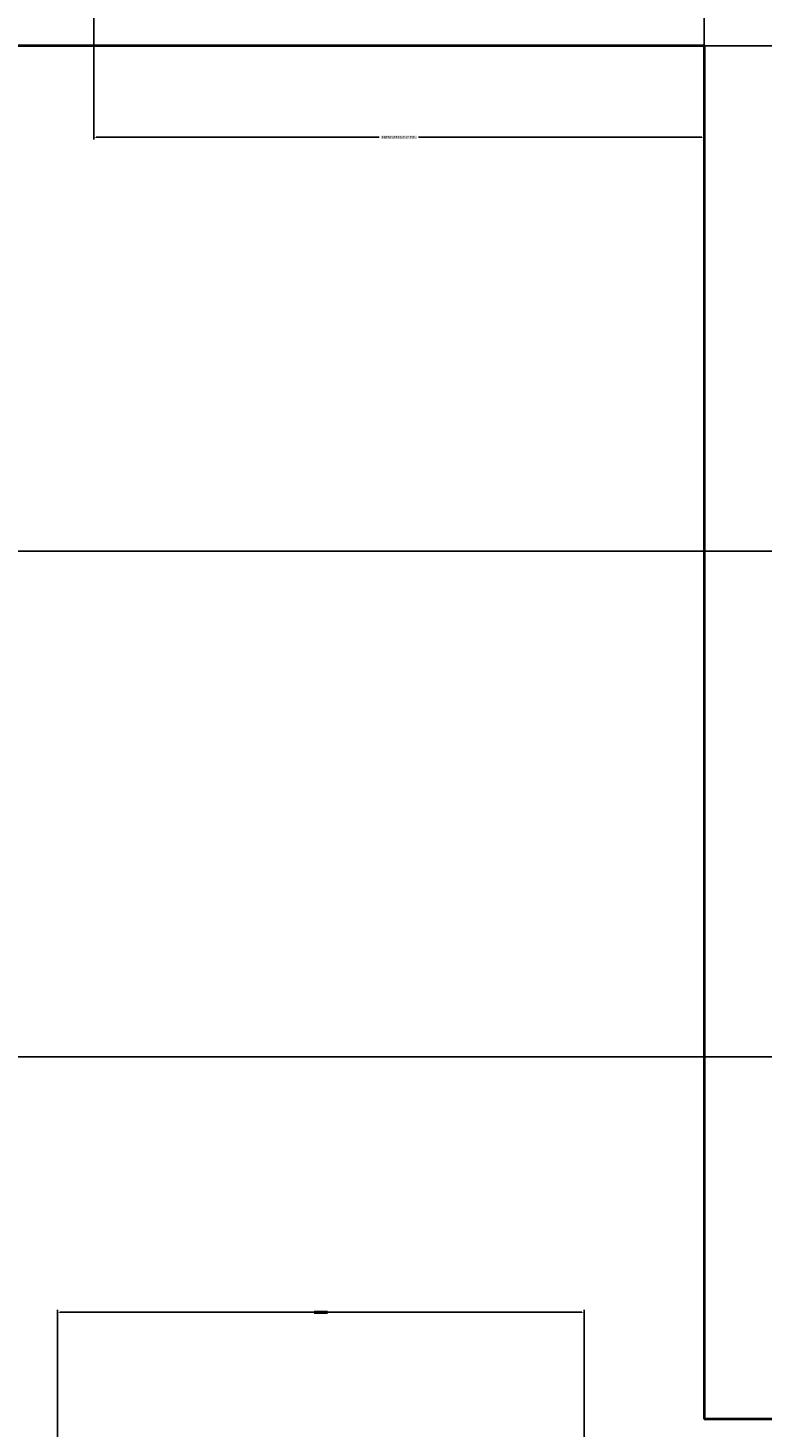
# Model space of a CAD drawing. Units: inches. Extents: x -301 to 715, y -607 to 364.
# Tile 117 of 141: x -43 to 14, y 192 to 303. Entities that reach past the tile are written whole.
import ezdxf

# ---------------------------------------------------------------- set-up
doc = ezdxf.new("R2010")
doc.units = ezdxf.units.IN
doc.header["$MEASUREMENT"] = 0
for name, color, linetype, lineweight in [('A-ANNO-DIMS', 2, 'Continuous', 18), ('A-FLOR-STRS', 2, 'Continuous', 25), ('A-WALL', 3, 'Continuous', 40)]:
    doc.layers.add(name, color=color, linetype=linetype, lineweight=lineweight)
doc.styles.get("Standard").update_dxf_attribs({"font": 'arial.ttf'})
doc.dimstyles.get("Standard").update_dxf_attribs({"dimtxt": 0.18, "dimasz": 0.18, "dimexe": 0.18, "dimexo": 0.0625, "dimgap": 0.09, "dimtad": 0, "dimtih": 1, "dimtoh": 1, "dimdec": 1, "dimzin": 0, "dimdsep": 46, "dimlunit": 4, "dimtxsty": 'Standard', "dimcen": 0.09, "dimclrd": 3, "dimclre": 4, "dimclrt": 6, "dimadec": 0, "dimazin": 0, "dimtfac": 1, "dimtdec": 1, "dimtofl": 0, "dimtmove": 0, "dimatfit": 3, "dimfxl": 1, "dimtfill": 2, "dimtfillclr": 51, "dimtolj": 1, "dimtzin": 0, "dimarcsym": 0})

# ---------------------------------------------------------------- blocks, each defined once
blk = doc.blocks.new('ENTRY-STEPS-48')
for p, q in [((0, 27), (0, 18)), ((48, 27), (48, 18)), ((0, 18), (0, 9)), ((48, 9), (48, 18)), ((0, 9), (48, 9)), ((0, 9), (0, 0)), ((48, 0), (48, 9)), ((0, 0), (48, 0))]:
    blk.add_line(p, q)
blk = doc.blocks.new('*D122')
at = {"layer": 'A-ANNO-DIMS', "color": 4, "lineweight": -2, "transparency": 16777216}
for p, q in [((-38.1, 301.12), (-38.1, 293.8)), ((9.9, 301.12), (9.9, 293.8))]:
    blk.add_line(p, q, dxfattribs=at)
at = {"layer": 'A-ANNO-DIMS', "color": 3, "lineweight": -2, "transparency": 16777216}
for p, q in [((-37.92, 293.98), (-15.65, 293.98)), ((9.72, 293.98), (-12.56, 293.98))]:
    blk.add_line(p, q, dxfattribs=at)
at = {"layer": 'A-ANNO-DIMS', "color": 3, "transparency": 16777216}
for points in [[(-37.92, 294.01), (-37.92, 293.95), (-38.1, 293.98)], [(9.72, 294.01), (9.72, 293.95), (9.9, 293.98)]]:
    blk.add_solid(points, dxfattribs=at)
at = {"layer": 'Defpoints', "color": 0, "transparency": 16777216}
for p in [(-38.1, 301.18), (9.9, 301.18), (-38.1, 293.98)]:
    blk.add_point(p, dxfattribs=at)
at = {"layer": 'A-ANNO-DIMS', "color": 6, "transparency": 16777216, "insert": (-14.1, 293.98), "char_height": 0.18, "attachment_point": 5, "bg_fill": 1, "box_fill_scale": 1.25, "bg_fill_color": 51, "bg_fill_transparency": 0}
blk.add_mtext('\\A1;ENTRY STEPS 4\'-0" TYP.', dxfattribs=at)
blk = doc.blocks.new('*D123')
at = {"layer": 'A-ANNO-DIMS', "color": 4, "lineweight": -2, "transparency": 16777216}
for p, q in [((9.96, 328.18), (17.28, 328.18)), ((9.96, 301.18), (17.28, 301.18))]:
    blk.add_line(p, q, dxfattribs=at)
at = {"layer": 'A-ANNO-DIMS', "color": 3, "lineweight": -2, "transparency": 16777216}
for p, q in [((17.1, 328), (17.1, 314.86)), ((17.1, 301.36), (17.1, 314.5))]:
    blk.add_line(p, q, dxfattribs=at)
at = {"layer": 'A-ANNO-DIMS', "color": 3, "transparency": 16777216}
for points in [[(17.07, 328), (17.13, 328), (17.1, 328.18)], [(17.07, 301.36), (17.13, 301.36), (17.1, 301.18)]]:
    blk.add_solid(points, dxfattribs=at)
at = {"layer": 'Defpoints', "color": 0, "transparency": 16777216}
for p in [(9.9, 328.18), (9.9, 301.18), (17.1, 301.18)]:
    blk.add_point(p, dxfattribs=at)
at = {"layer": 'A-ANNO-DIMS', "color": 6, "transparency": 16777216, "insert": (17.1, 314.68), "char_height": 0.18, "attachment_point": 5, "bg_fill": 1, "box_fill_scale": 1.25, "bg_fill_color": 51, "bg_fill_transparency": 0}
blk.add_mtext('\\A1;2\'-3" TYP.', dxfattribs=at)
blk = doc.blocks.new('*D129')
at = {"layer": 'A-ANNO-DIMS', "color": 4, "lineweight": -2, "transparency": 16777216}
for p, q in [((-40.96, 191.37), (-40.96, 201.77)), ((0.47, 191.37), (0.47, 201.77))]:
    blk.add_line(p, q, dxfattribs=at)
at = {"layer": 'A-ANNO-DIMS', "color": 3, "lineweight": -2, "transparency": 16777216}
for p, q in [((-40.78, 201.59), (-20.78, 201.59)), ((0.29, 201.59), (-19.71, 201.59))]:
    blk.add_line(p, q, dxfattribs=at)
at = {"layer": 'A-ANNO-DIMS', "color": 3, "transparency": 16777216}
for points in [[(-40.78, 201.62), (-40.78, 201.56), (-40.96, 201.59)], [(0.29, 201.62), (0.29, 201.56), (0.47, 201.59)]]:
    blk.add_solid(points, dxfattribs=at)
at = {"layer": 'Defpoints', "color": 0, "transparency": 16777216}
for p in [(-40.96, 201.59), (-40.96, 191.31), (0.47, 191.31)]:
    blk.add_point(p, dxfattribs=at)
at = {"layer": 'A-ANNO-DIMS', "color": 6, "transparency": 16777216, "insert": (-20.24, 201.59), "char_height": 0.18, "attachment_point": 5, "bg_fill": 1, "box_fill_scale": 1.25, "bg_fill_color": 51, "bg_fill_transparency": 0}
blk.add_mtext('\\A1;3\'-5 1/2"', dxfattribs=at)
blk = doc.blocks.new('*D157')
at = {"layer": 'A-ANNO-DIMS', "color": 4, "lineweight": -2, "transparency": 16777216}
for p, q in [((-50.54, 261.43), (233.66, 261.43)), ((-50.54, 221.68), (233.66, 221.68))]:
    blk.add_line(p, q, dxfattribs=at)
at = {"layer": 'A-ANNO-DIMS', "color": 3, "lineweight": -2, "transparency": 16777216}
for p, q in [((233.48, 261.25), (233.48, 241.74)), ((233.48, 221.86), (233.48, 241.38))]:
    blk.add_line(p, q, dxfattribs=at)
at = {"layer": 'A-ANNO-DIMS', "color": 3, "transparency": 16777216}
for points in [[(233.45, 261.25), (233.51, 261.25), (233.48, 261.43)], [(233.45, 221.86), (233.51, 221.86), (233.48, 221.68)]]:
    blk.add_solid(points, dxfattribs=at)
at = {"layer": 'Defpoints', "color": 0, "transparency": 16777216}
for p in [(-50.6, 261.43), (233.48, 261.43), (-50.6, 221.68)]:
    blk.add_point(p, dxfattribs=at)
at = {"layer": 'A-ANNO-DIMS', "color": 6, "transparency": 16777216, "insert": (233.48, 241.56), "char_height": 0.18, "attachment_point": 5, "bg_fill": 1, "box_fill_scale": 1.25, "bg_fill_color": 51, "bg_fill_transparency": 0}
blk.add_mtext('\\A1;3\'-4"', dxfattribs=at)

msp = doc.modelspace()

# ---------------------------------------------------------------- linework, layer by layer
at = {"layer": 'A-WALL'}
for p, q in [((9.9, 301.18), (-195.6, 301.18)), ((9.9, 301.18), (9.9, 193.18)), ((15.9, 193.18), (9.9, 193.18))]:
    msp.add_line(p, q, dxfattribs=at)

# ---------------------------------------------------------------- block references
at = {"layer": 'A-FLOR-STRS', "rotation": 180}
msp.add_blockref('ENTRY-STEPS-48', (9.9, 328.18), dxfattribs=at)

# ---------------------------------------------------------------- dimensions: what is measured, and where the dimension line sits
at = {"layer": 'A-ANNO-DIMS'}
for base, p1, p2, angle, text, picture, middle in [((17.1, 301.18), (9.9, 328.18), (9.9, 301.18), 270, '<> TYP.', '*D123', (17.1, 314.68)), ((-38.1, 293.98), (9.9, 301.18), (-38.1, 301.18), 180, 'ENTRY STEPS <> TYP.', '*D122', (-14.1, 293.98))]:
    dim = msp.add_linear_dim(base=base, p1=p1, p2=p2, angle=angle, text=text, dimstyle='Standard', override={"dimdec": 1, "dimlfac": 1, "dimrnd": 0, "dimzin": 1, "dimdsep": 46, "dimlunit": 4, "dimfrac": 2}, dxfattribs=at)
    dim.commit()
    dim.dimension.update_dxf_attribs({"geometry": picture, "text_midpoint": middle})
for base, p1, p2, angle, picture, middle in [((233.479242, 261.43233), (-50.603288, 221.68233), (-50.603288, 261.43233), 90, '*D157', (233.479242, 241.55733)), ((-40.96, 201.59), (0.47, 191.31), (-40.96, 191.31), 180, '*D129', (-20.24, 201.59))]:
    dim = msp.add_linear_dim(base=base, p1=p1, p2=p2, angle=angle, dimstyle='Standard', override={"dimdec": 1, "dimlfac": 1, "dimrnd": 0, "dimzin": 1, "dimdsep": 46, "dimlunit": 4, "dimfrac": 2}, dxfattribs=at)
    dim.commit()
    dim.dimension.update_dxf_attribs({"geometry": picture, "text_midpoint": middle})

doc.saveas('drawing.dxf')
